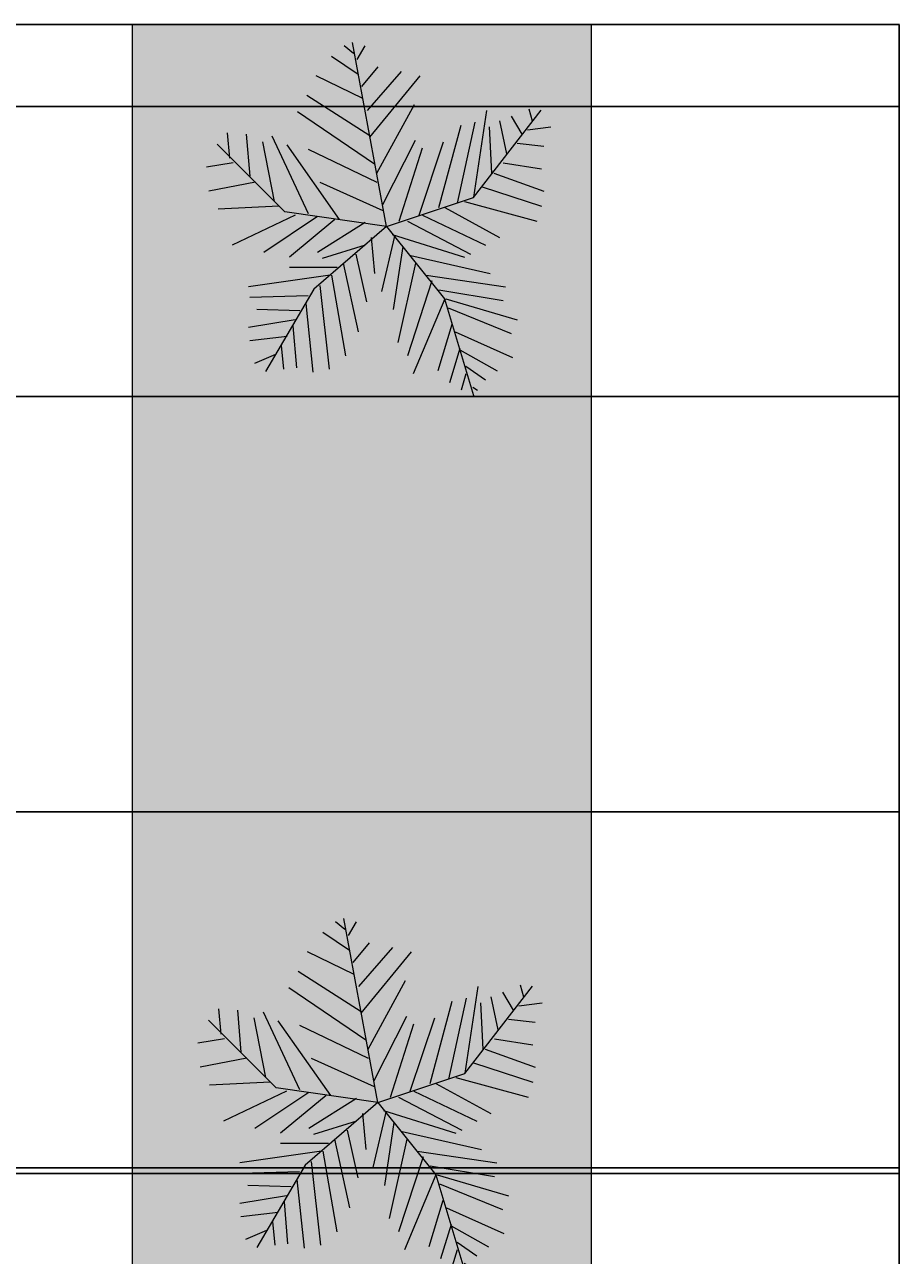
# Model space of a CAD drawing. Units: millimetres. Extents: x -229 to 16545, y -10488 to 4272.
# Tile 29 of 29: x 14086 to 16545, y -1208 to 2252. Entities that reach past the tile are written whole.
import ezdxf

# ---------------------------------------------------------------- set-up
doc = ezdxf.new("R2010")
doc.units = ezdxf.units.MM
for name, color, linetype, lineweight in [('A-ANNO-DIMS', 2, 'Continuous', 18), ('L-PLNT-BEDS', 82, 'Continuous', 18), ('L-PLNT-TREE', 80, 'Continuous', 18)]:
    doc.layers.add(name, color=color, linetype=linetype, lineweight=lineweight)
doc.layers.add('L-PLNT-PATT', color=116, linetype='Continuous', lineweight=13, true_color=0x136734)
doc.styles.get("Standard").update_dxf_attribs({"font": 'arial.ttf'})
doc.dimstyles.get("Standard").update_dxf_attribs({"dimtxt": 0.18, "dimasz": 0.18, "dimexe": 0.18, "dimexo": 0.0625, "dimgap": 0.09, "dimtad": 0, "dimtih": 1, "dimtoh": 1, "dimdec": 4, "dimzin": 0, "dimdsep": 46, "dimtxsty": 'Standard', "dimcen": 0.09, "dimadec": 0, "dimazin": 0, "dimtfac": 1, "dimtdec": 4, "dimtofl": 0, "dimtmove": 0, "dimatfit": 3, "dimfxl": 1, "dimtolj": 1, "dimtzin": 0, "dimarcsym": 0})

# ---------------------------------------------------------------- blocks, each defined once
blk = doc.blocks.new('*U18')
for p, q in [((-10.186, 53.64), (-13.084, 55.962)), ((0, 0), (-10.5, 57)), ((-9.099, 51.782), (-6.563, 55.962)), ((-8.737, 47.138), (-17.069, 52.711)), ((-7.288, 39.707), (-21.778, 46.673)), ((-7.65, 43.423), (-2.578, 49.46)), ((-5.839, 35.992), (4.667, 48.067)), ((-5.114, 27.632), (10.463, 46.673)), ((-5.114, 28.097), (-24.676, 40.636)), ((-3.665, 19.273), (-27.574, 35.527)), ((-2.941, 16.486), (8.652, 37.85)), ((27, 9), (48, 36)), ((27.127, 9.056), (31.112, 35.992)), ((44.153, 36.456), (45.239, 32.741)), ((16.259, 5.805), (23.142, 31.348)), ((22.055, 7.198), (27.489, 32.277)), ((31.836, 30.883), (32.561, 16.486)), ((35.096, 32.741), (37.27, 22.524)), ((38.719, 34.134), (41.979, 28.561)), ((43.791, 29.954), (51.036, 30.883)), ((-48.585, 21.131), (-49.309, 29.026)), ((-43.513, 28.561), (-42.427, 15.558)), ((-35.544, 28.097), (-24.314, 3.947)), ((-31.5, 4.5), (-52.5, 25.5)), ((-38.442, 26.239), (-34.819, 7.663)), ((-14.533, 2.09), (-30.834, 25.31)), ((-24.314, 23.917), (-2.941, 13.7)), ((-1.129, 6.734), (9.014, 26.704)), ((3.942, 1.625), (11.187, 24.381)), ((10.101, 3.483), (17.708, 26.239)), ((40.53, 25.775), (48.862, 24.846)), ((-47.498, 19.737), (-55.83, 18.344)), ((36.183, 19.737), (48.137, 17.88)), ((33.285, 16.486), (48.862, 10.913)), ((-40.615, 13.7), (-55.105, 10.913)), ((-20.691, 13.7), (-1.129, 4.876)), ((29.662, 12.307), (48.137, 6.269)), ((0, 0), (27, 9)), ((24.229, 7.663), (46.688, 1.625)), ((-33.37, 6.269), (-52.207, 5.34)), ((0, 0), (-31.5, 4.5)), ((18.07, 5.805), (35.096, -3.483)), ((-28.299, 3.483), (-47.86, -5.805)), ((-21.416, 3.018), (-38.079, -8.128)), ((-15.982, 2.09), (-30.11, -9.521)), ((0, 0), (-22.5, -19.5)), ((-6.563, 1.161), (-21.416, -8.128)), ((0, 0), (18, -22.5)), ((6.478, 1.625), (26.04, -8.592)), ((11.187, 3.483), (30.749, -5.805)), ((-4.752, -3.483), (-3.665, -14.629)), ((2.493, -3.019), (-1.491, -20.202)), ((1.769, -2.555), (24.229, -9.521)), ((-6.563, -5.805), (-19.967, -9.985)), ((5.029, -6.27), (2.131, -25.775)), ((-13.446, -11.378), (-8.737, -32.741)), ((-9.461, -8.592), (-6.201, -23.453)), ((9.014, -11.378), (3.58, -35.992)), ((7.565, -9.056), (32.198, -14.629)), ((-17.431, -15.094), (-42.789, -18.809)), ((-15.257, -12.772), (-30.11, -12.772)), ((-17.069, -15.094), (-12.721, -40.172)), ((12.274, -15.094), (36.907, -18.809)), ((-20.691, -18.345), (-17.793, -44.352)), ((14.085, -16.951), (6.478, -40.172)), ((-24.314, -21.596), (-42.427, -22.06)), ((-22.5, -19.5), (-37.5, -45)), ((18.07, -22.524), (8.289, -45.745)), ((16.259, -19.738), (36.183, -22.989)), ((18, -22.5), (27, -52.5)), ((18.433, -22.524), (40.53, -29.026)), ((-26.849, -26.24), (-40.253, -25.775)), ((-25.038, -23.918), (-22.865, -45.281)), ((19.157, -25.311), (38.719, -33.206)), ((-28.299, -29.026), (-42.789, -31.348)), ((20.244, -30.419), (15.897, -44.816)), ((-30.834, -34.135), (-42.427, -35.528)), ((-29.023, -30.884), (-27.936, -43.887)), ((21.331, -32.741), (39.081, -40.636)), ((-32.646, -36.921), (-31.921, -44.352)), ((22.78, -37.85), (19.519, -48.532)), ((-34.457, -39.708), (-40.978, -42.494)), ((22.78, -38.314), (34.372, -44.816)), ((24.591, -45.745), (23.142, -50.854)), ((24.591, -43.423), (30.749, -47.603)), ((26.764, -49.925), (28.213, -50.854))]:
    blk.add_line(p, q)
blk = doc.blocks.new('*D48')
at = {"layer": 'A-ANNO-DIMS', "color": 0, "lineweight": -2, "transparency": 16777216}
for p, q in [((14016, 2251.7), (16544.5, 2251.7)), ((16544.3, 2251.5), (16544.3, -1593.1)), ((16544.3, -5438.1), (16544.3, -1593.5)), ((13786, -5438.3), (16544.5, -5438.3))]:
    blk.add_line(p, q, dxfattribs=at)
at = {"layer": 'A-ANNO-DIMS', "color": 0, "transparency": 16777216}
for points in [[(16544.3, 2251.5), (16544.4, 2251.5), (16544.3, 2251.7)], [(16544.3, -5438.1), (16544.4, -5438.1), (16544.3, -5438.3)]]:
    blk.add_solid(points, dxfattribs=at)
at = {"layer": 'Defpoints', "color": 0, "transparency": 16777216}
for p in [(14015.9, 2251.7), (13785.9, -5438.3), (16544.3, -5438.3)]:
    blk.add_point(p, dxfattribs=at)
at = {"layer": 'A-ANNO-DIMS', "color": 0, "transparency": 16777216, "insert": (16544.3, -1593.3), "char_height": 0.18, "attachment_point": 5}
blk.add_mtext('\\A1;7690', dxfattribs=at)
blk = doc.blocks.new('*D65')
at = {"layer": 'A-ANNO-DIMS', "color": 0, "lineweight": -2, "transparency": 16777216}
for p, q in [((13786, 2021.7), (16544.5, 2021.7)), ((16544.3, 2021.5), (16544.3, 521.9)), ((16544.3, -978.1), (16544.3, 521.5)), ((13786, -978.3), (16544.5, -978.3))]:
    blk.add_line(p, q, dxfattribs=at)
at = {"layer": 'A-ANNO-DIMS', "color": 0, "transparency": 16777216}
for points in [[(16544.3, 2021.5), (16544.4, 2021.5), (16544.3, 2021.7)], [(16544.3, -978.1), (16544.4, -978.1), (16544.3, -978.3)]]:
    blk.add_solid(points, dxfattribs=at)
at = {"layer": 'Defpoints', "color": 0, "transparency": 16777216}
for p in [(13785.9, 2021.7), (13785.9, -978.3), (16544.3, -978.3)]:
    blk.add_point(p, dxfattribs=at)
at = {"layer": 'A-ANNO-DIMS', "color": 0, "transparency": 16777216, "insert": (16544.3, 521.7), "char_height": 0.18, "attachment_point": 5}
blk.add_mtext('\\A1;3000', dxfattribs=at)
blk = doc.blocks.new('*D66')
at = {"layer": 'A-ANNO-DIMS', "color": 0, "lineweight": -2, "transparency": 16777216}
for p, q in [((9556, 38.2), (16544.5, 38.2)), ((16544.3, 38), (16544.3, -461.6)), ((16544.3, -961.6), (16544.3, -462)), ((9556, -961.8), (16544.5, -961.8))]:
    blk.add_line(p, q, dxfattribs=at)
at = {"layer": 'A-ANNO-DIMS', "color": 0, "transparency": 16777216}
for points in [[(16544.3, 38), (16544.4, 38), (16544.3, 38.2)], [(16544.3, -961.6), (16544.4, -961.6), (16544.3, -961.8)]]:
    blk.add_solid(points, dxfattribs=at)
at = {"layer": 'Defpoints', "color": 0, "transparency": 16777216}
for p in [(9555.9, 38.2), (9555.9, -961.8), (16544.3, -961.8)]:
    blk.add_point(p, dxfattribs=at)
at = {"layer": 'A-ANNO-DIMS', "color": 0, "transparency": 16777216, "insert": (16544.3, -461.8), "char_height": 0.18, "attachment_point": 5}
blk.add_mtext('\\A1;1000', dxfattribs=at)
blk = doc.blocks.new('*D99')
at = {"layer": 'A-ANNO-DIMS', "color": 0, "lineweight": -2, "transparency": 16777216}
for p, q in [((13786, 2021.7), (16544.5, 2021.7)), ((16544.3, 2021.5), (16544.3, 1614.4)), ((16544.3, 1206.9), (16544.3, 1614)), ((13723, 1206.7), (16544.5, 1206.7))]:
    blk.add_line(p, q, dxfattribs=at)
at = {"layer": 'A-ANNO-DIMS', "color": 0, "transparency": 16777216}
for points in [[(16544.3, 2021.5), (16544.4, 2021.5), (16544.3, 2021.7)], [(16544.3, 1206.9), (16544.4, 1206.9), (16544.3, 1206.7)]]:
    blk.add_solid(points, dxfattribs=at)
at = {"layer": 'Defpoints', "color": 0, "transparency": 16777216}
for p in [(13785.9, 2021.7), (13722.9, 1206.7), (16544.3, 1206.7)]:
    blk.add_point(p, dxfattribs=at)
at = {"layer": 'A-ANNO-DIMS', "color": 0, "transparency": 16777216, "insert": (16544.3, 1614.2), "char_height": 0.18, "attachment_point": 5}
blk.add_mtext('\\A1;815', dxfattribs=at)

msp = doc.modelspace()

# ---------------------------------------------------------------- hatches: boundary and pattern name
at = {"layer": 'L-PLNT-PATT'}
h = msp.add_hatch(dxfattribs=at)
h.set_pattern_fill('GRASS', color=256, scale=2)
h.set_pattern_definition([(90, (-8141.222, -13125.504), (-35.921024, 35.921024), [9.525, -62.31705]), (45, (-8141.22, -13125.504), (-35.92102, 35.92102), [9.525, -41.275]), (135, (-8141.22, -13125.504), (-35.92102, -35.92102), [9.525, -41.275])])
h.paths.add_polyline_path([(15679.607, 2251.728), (14387.79, 2251.728), (14387.79, -7668.272), (8209.16, -7668.272), (8209.16, -9248.272), (14015.933, -9248.272), (15679.607, -9248.272)])

# ---------------------------------------------------------------- linework, layer by layer
at = {"layer": 'L-PLNT-BEDS', "transparency": 33554554}
for p, q in [((15679.607, 2251.728), (14387.79, 2251.728)), ((15679.607, -9248.272), (15679.607, 2251.728))]:
    msp.add_line(p, q, dxfattribs=at)
at = {"layer": 'L-PLNT-BEDS', "transparency": 33554572}
msp.add_line((14387.79, 2251.728), (14387.79, -7668.272), dxfattribs=at)

# ---------------------------------------------------------------- block references
at = {"layer": 'L-PLNT-TREE', "xscale": 9.061891725250485, "yscale": 9.061891725250485, "zscale": 9.061891725250485}
for p in [(15102.87, 1684.576), (15078.323, -778.078)]:
    msp.add_blockref('*U18', p, dxfattribs=at)

# ---------------------------------------------------------------- dimensions: what is measured, and where the dimension line sits
at = {"layer": 'A-ANNO-DIMS'}
for base, p1, p2, picture, middle in [((16544.342, -5438.272), (14015.933, 2251.728), (13785.933, -5438.272), '*D48', (16544.342, -1593.272)), ((16544.342, 1206.716), (13785.933, 2021.728), (13722.905, 1206.716), '*D99', (16544.342, 1614.222)), ((16544.342, -978.272), (13785.933, 2021.728), (13785.933, -978.272), '*D65', (16544.342, 521.728)), ((16544.342, -961.785), (9555.933, 38.215), (9555.933, -961.785), '*D66', (16544.342, -461.785))]:
    dim = msp.add_linear_dim(base=base, p1=p1, p2=p2, angle=90, dimstyle='Standard', override={"dimdec": 0, "dimlfac": 1, "dimrnd": 0, "dimzin": 0, "dimdsep": 46, "dimlunit": 2}, dxfattribs=at)
    dim.commit()
    dim.dimension.update_dxf_attribs({"geometry": picture, "text_midpoint": middle})

doc.saveas('drawing.dxf')
